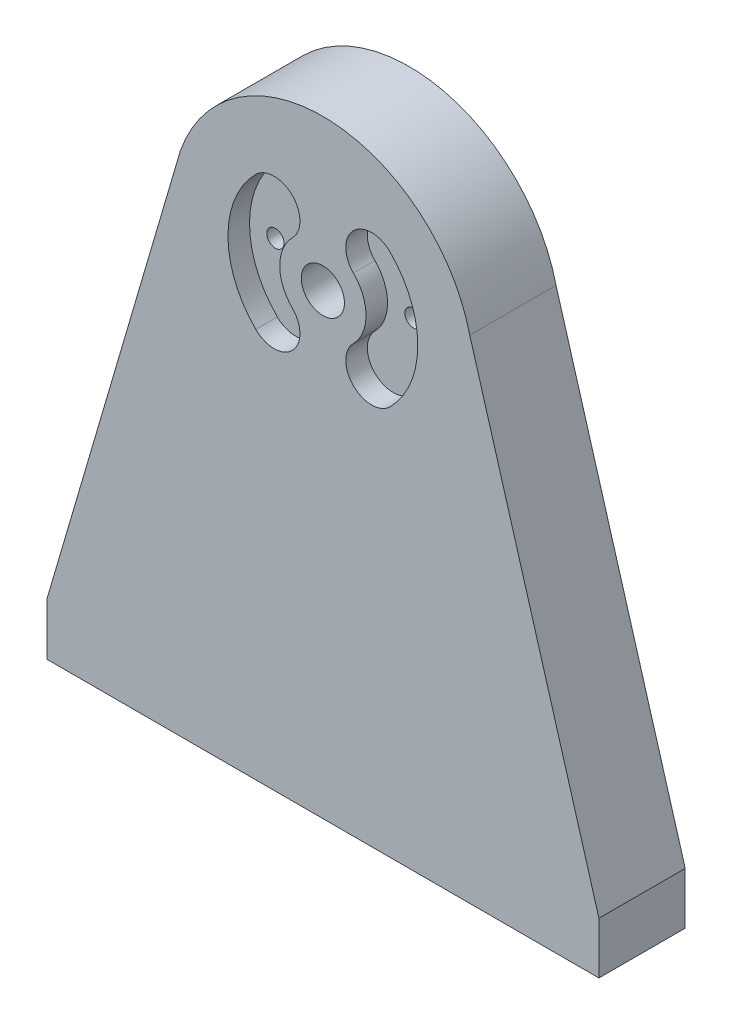
from build123d import *

# Parameters (mm, degrees)
POST_PLATE_10MM_DEPTH       = 10
UPPER_SLOT_PROFILE_R        = 2.5
UPPER_SLOT_CUT_DEPTH        = 10
UPPER_SLOT_RELIEF_PROFILE_R = 2.1
UPPER_SLOT_RELIEF_CUT_DEPTH = 12.4
LONG_SLOT_PROFILE_R         = 1
LONG_SLOT_CUT_55_DEEP_DEPTH = 55
SHAFT_BORE_5_PROFILE_R      = 2.5
SHAFT_BORE_5_DEPTH          = 55
PIVOT_RECESS_2_5_DEEP_DEPTH = 2.5
LOWER_SLOT_PROFILE_R        = 1
LOWER_SLOT_CUT_DEPTH        = 5


with BuildPart() as part:
    # Post Plate Profile → Post Plate 10mm (new body)
    with BuildSketch(Plane.XY):
        with BuildLine():
            Line((-32, 0), (32, 0))
            Line((32, 0), (32, 6))
            Line((32, 6), (17.027168619, 57.040486211))
            ThreePointArc((17.027168619, 57.040486211), (0.915873878, 70.476017139), (-16.511549747, 58.798165653))
            Line((-16.511549747, 58.798165653), (-32, 6))
            Line((-32, 6), (-32, 0))
        make_face()
    extrude(amount=POST_PLATE_10MM_DEPTH)

    # Upper Slot Profile → Upper Slot Cut (cut)
    with BuildSketch(Plane.XZ):
        with Locations(Location((22, 5, 0), (0, 0, 270))):
            Circle(UPPER_SLOT_PROFILE_R)
        with Locations(Location((-22, 5, 0), (0, 0, 270))):
            Circle(UPPER_SLOT_PROFILE_R)
    extrude(amount=-UPPER_SLOT_CUT_DEPTH, mode=Mode.SUBTRACT)

    # Upper Slot Relief Profile → Upper Slot Relief Cut (cut)
    with BuildSketch(Plane.XZ):
        with Locations(Location((22, 5, 0), (0, 0, 270))):
            Circle(UPPER_SLOT_RELIEF_PROFILE_R)
        with Locations(Location((-22, 5, 0), (0, 0, 270))):
            Circle(UPPER_SLOT_RELIEF_PROFILE_R)
    extrude(amount=-UPPER_SLOT_RELIEF_CUT_DEPTH, mode=Mode.SUBTRACT)

    # Long Slot Profile → Long Slot Cut 55 Deep (cut)
    with BuildSketch(Plane.XZ):
        with Locations(Location((-8, 5, 0), (0, 0, 270))):
            Circle(LONG_SLOT_PROFILE_R)
        with Locations(Location((8, 5, 0), (0, 0, 270))):
            Circle(LONG_SLOT_PROFILE_R)
    extrude(amount=-LONG_SLOT_CUT_55_DEEP_DEPTH, mode=Mode.SUBTRACT)

    # Shaft Bore Ø5 Profile → Shaft Bore Ø5 (cut)
    with BuildSketch(Plane.XY.offset(10)):
        with Locations((0, 53)):
            Circle(SHAFT_BORE_5_PROFILE_R)
    extrude(amount=-SHAFT_BORE_5_DEPTH, mode=Mode.SUBTRACT)

    # Pivot Recess Profile → Pivot Recess 2.5 Deep (cut)
    with BuildSketch(Plane.XY.offset(10)):
        with BuildLine():
            ThreePointArc((-3.535533906, 56.535533906), (-5, 53), (-3.535533906, 49.464466094))
            ThreePointArc((-3.535533906, 49.464466094), (-3.535533906, 45.221825407), (-7.778174593, 45.221825407))
            ThreePointArc((-7.778174593, 45.221825407), (-11, 53), (-7.778174593, 60.778174593))
            ThreePointArc((-7.778174593, 60.778174593), (-3.535533906, 60.778174593), (-3.535533906, 56.535533906))
        make_face()
        with BuildLine():
            ThreePointArc((7.778174593, 45.221825407), (11, 53), (7.778174593, 60.778174593))
            ThreePointArc((7.778174593, 60.778174593), (3.535533906, 60.778174593), (3.535533906, 56.535533906))
            ThreePointArc((3.535533906, 56.535533906), (5, 53), (3.535533906, 49.464466094))
            ThreePointArc((3.535533906, 49.464466094), (3.535533906, 45.221825407), (7.778174593, 45.221825407))
        make_face()
    extrude(amount=-PIVOT_RECESS_2_5_DEEP_DEPTH, mode=Mode.SUBTRACT)

    # Lower Slot Profile → Lower Slot Cut (cut)
    with BuildSketch(Plane.XY.offset(7.5)):
        with Locations((8, 53)):
            Circle(LOWER_SLOT_PROFILE_R)
        with Locations((-8, 53)):
            Circle(LOWER_SLOT_PROFILE_R)
    extrude(amount=-LOWER_SLOT_CUT_DEPTH, mode=Mode.SUBTRACT)


solid = part.part
